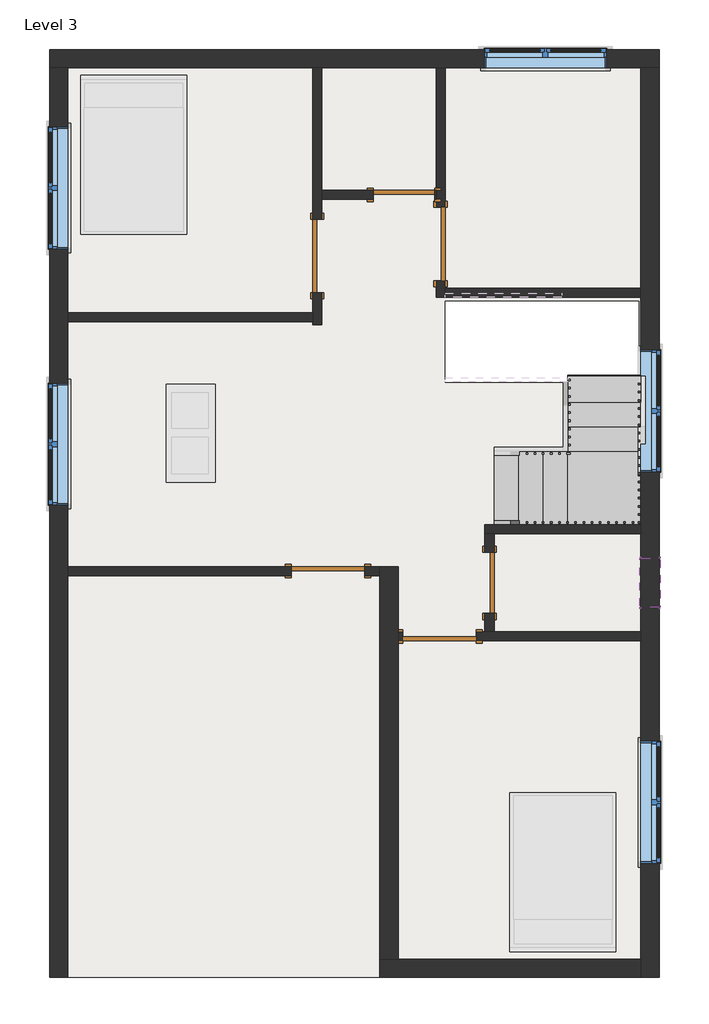
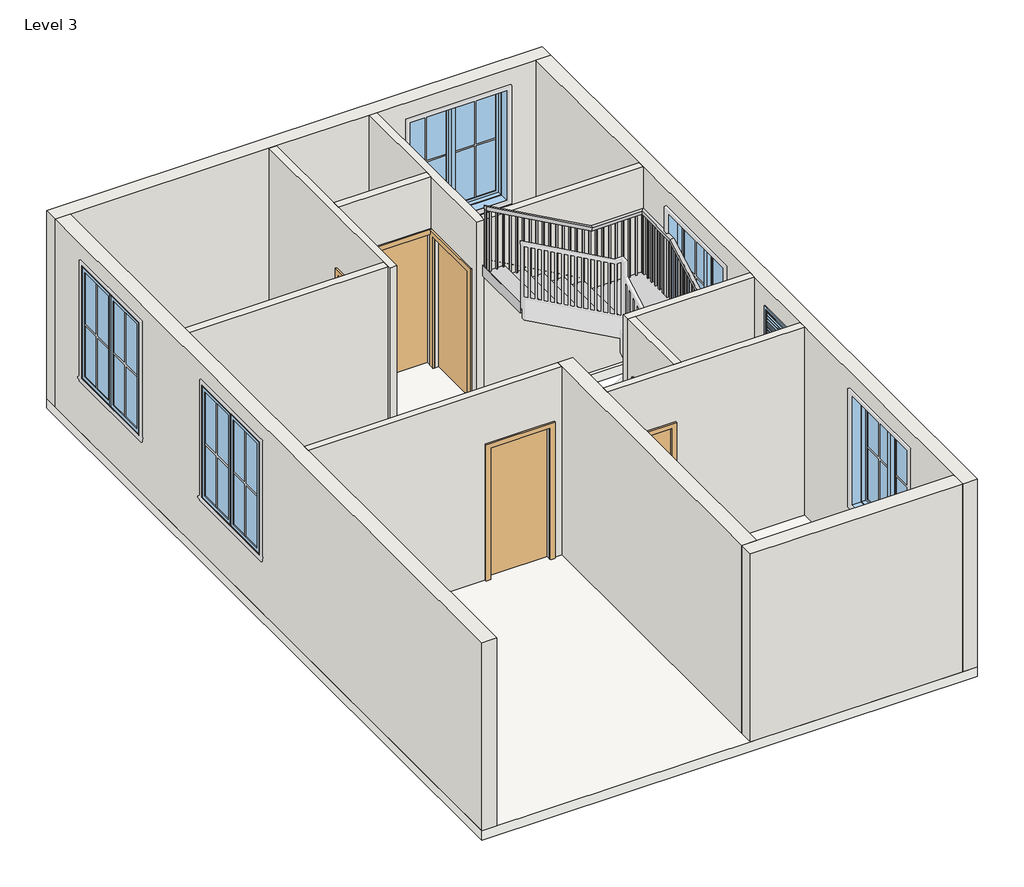
# One storey, part 1 of 2: 14 walls, 6 doors, 6 windows, 1 railing, 1 slab, 1 stair flight.
"""IFC4 building model written with IfcOpenShell, lengths in millimetres."""

from ifc_helpers import new_model, si_unit, frame, origin, place, context, project, spatial, polyline, outline, extrude, faceted_brep, transform, mapped, element, save
from components import door_214872d5, door_78caadf7, single_flush_door_3_e5f9f3c4, single_flush_door_3_305aa2a5, stair_flight_3451e034, window_casement_double_win_5_f93960c7, window_f2d8fef0

model = new_model("IFC4")

# Units and contexts
model_context = context("Model", 3, world=origin())
ifc_project = project(units=[si_unit("LENGTHUNIT", "METRE", prefix="MILLI")], contexts=[model_context])

# Site, building, storey
site = spatial("IfcSite", under=ifc_project)
building = spatial("IfcBuilding", under=site)
storey = spatial("IfcBuildingStorey", under=building, Name="Level 3", Elevation=3200.4)

# Doors
placement = place(None, origin())
door_shape = door_214872d5(model_context)
element("IfcDoor", 1, ObjectType="Single-Flush : DOOR 2'6\"", at=placement, inside=storey, context=model_context, shape_type="MappedRepresentation", body=[
    mapped(door_shape, transform((-185.4325206, 3926.3629493, 3200.4), x_axis=(1.0, 0.0, 0.0), y_axis=(0.0, 1.0, 0.0), z_axis=(0.0, 0.0, 1.0))),
])
door_2_shape = door_78caadf7(model_context)
element("IfcDoor", 2, ObjectType="Single-Flush : DOOR 2'6\"", at=placement, inside=storey, context=model_context, shape_type="MappedRepresentation", body=[
    mapped(door_2_shape, transform((881.3674794, -905.9870507, 3200.4), x_axis=(0.0, 1.0, 0.0), y_axis=(-1.0, 0.0, 0.0), z_axis=(0.0, 0.0, 1.0))),
])
single_flush_door_3_shape = single_flush_door_3_e5f9f3c4(model_context)
element("IfcDoor", 3, ObjectType="Single-Flush : DOOR 3'", at=placement, inside=storey, context=model_context, shape_type="MappedRepresentation", body=[
    mapped(single_flush_door_3_shape, transform((271.7674794, 3316.7629493, 3200.4), x_axis=(0.0, -1.0, 0.0), y_axis=(1.0, 0.0, 0.0), z_axis=(0.0, 0.0, 1.0))),
])
element("IfcDoor", 4, ObjectType="Single-Flush : DOOR 3'", at=placement, inside=storey, context=model_context, shape_type="MappedRepresentation", body=[
    mapped(single_flush_door_3_shape, transform((255.8924794, -1572.7370507, 3200.4), x_axis=(-1.0, 0.0, 0.0), y_axis=(0.0, -1.0, 0.0), z_axis=(0.0, 0.0, 1.0))),
])
single_flush_door_3_2_shape = single_flush_door_3_305aa2a5(model_context)
element("IfcDoor", 5, ObjectType="Single-Flush : DOOR 3'", at=placement, inside=storey, context=model_context, shape_type="MappedRepresentation", body=[
    mapped(single_flush_door_3_2_shape, transform((-1264.9325206, 3164.3629493, 3200.4), x_axis=(0.0, -1.0, 0.0), y_axis=(1.0, 0.0, 0.0), z_axis=(0.0, 0.0, 1.0))),
])
element("IfcDoor", 6, ObjectType="Single-Flush : DOOR 3'6\"", at=placement, inside=storey, context=model_context, shape_type="MappedRepresentation", body=[
    mapped(single_flush_door_3_shape, transform((-1131.5825206, -759.9370507, 3200.4), x_axis=(1.0, 0.0, 0.0), y_axis=(0.0, 1.0, 0.0), z_axis=(0.0, 0.0, 1.0))),
])

# Railing
element("IfcRailing", 7, ObjectType="Handrail - Rectangular", at=placement, inside=storey, context=model_context, shape_type="SolidModel", body=[
    faceted_brep([(938.5174794, -131.2870507, 4284.1333333), (938.5174794, -131.2870507, 4226.020221), (938.5174794, -182.0870507, 4226.020221), (938.5174794, -182.0870507, 4284.1333333), (2005.3174794, -131.2870507, 4876.8), (2018.4810817, -131.2870507, 4826.0), (2018.4810817, -182.0870507, 4826.0), (2005.3174794, -182.0870507, 4876.8), (2716.5174794, -131.2870507, 4876.8), (2716.5174794, -131.2870507, 4826.0), (2767.3174794, -182.0870507, 4826.0), (2767.3174794, -182.0870507, 4876.8), (2716.5174794, 579.9129493, 4876.8), (2716.5174794, 593.0765516, 4826.0), (2767.3174794, 593.0765516, 4826.0), (2767.3174794, 579.9129493, 4876.8), (2716.5174794, 1843.5629493, 5578.8277778), (2716.5174794, 1856.7265516, 5528.0277778), (2767.3174794, 1856.7265516, 5528.0277778), (2767.3174794, 1843.5629493, 5578.8277778), (2716.5174794, 2599.2129493, 5578.8277778), (2716.5174794, 2599.2129493, 5528.0277778), (2767.3174794, 2650.0129493, 5528.0277778), (2767.3174794, 2650.0129493, 5578.8277778), (1960.8674794, 2599.2129493, 5578.8277778), (1947.7038772, 2599.2129493, 5528.0277778), (1947.7038772, 2650.0129493, 5528.0277778), (1960.8674794, 2650.0129493, 5578.8277778), (328.9174794, 2599.2129493, 6485.4666667), (328.9174794, 2650.0129493, 6485.4666667), (328.9174794, 2650.0129493, 6427.3535543), (328.9174794, 2599.2129493, 6427.3535543)], [[[0, 1, 2, 3]], [[1, 0, 4, 5]], [[2, 1, 5, 6]], [[3, 2, 6, 7]], [[0, 3, 7, 4]], [[5, 4, 8, 9]], [[6, 5, 9, 10]], [[7, 6, 10, 11]], [[4, 7, 11, 8]], [[9, 8, 12, 13]], [[10, 9, 13, 14]], [[11, 10, 14, 15]], [[8, 11, 15, 12]], [[13, 12, 16, 17]], [[14, 13, 17, 18]], [[15, 14, 18, 19]], [[12, 15, 19, 16]], [[17, 16, 20, 21]], [[18, 17, 21, 22]], [[19, 18, 22, 23]], [[16, 19, 23, 20]], [[21, 20, 24, 25]], [[22, 21, 25, 26]], [[23, 22, 26, 27]], [[20, 23, 27, 24]], [[28, 29, 30, 31]], [[25, 24, 28, 31]], [[26, 25, 31, 30]], [[27, 26, 30, 29]], [[24, 27, 29, 28]]]),
    extrude(outline(polyline([(6379.7285543, 414.6424794), (6390.3118876, 395.5924794), (5401.7333333, 395.5924794), (5401.7333333, 414.6424794), (6379.7285543, 414.6424794)])), frame((0.0, 2615.0879493, 0.0), z_axis=(0.0, 1.0, 0.0), x_axis=(0.0, 0.0, 1.0)), (0.0, 0.0, 1.0), 19.05),
    extrude(outline(polyline([(6323.2841099, 516.2424794), (6333.8674432, 497.1924794), (5401.7333333, 497.1924794), (5401.7333333, 516.2424794), (6323.2841099, 516.2424794)])), frame((0.0, 2615.0879493, 0.0), z_axis=(0.0, 1.0, 0.0), x_axis=(0.0, 0.0, 1.0)), (0.0, 0.0, 1.0), 19.05),
    extrude(outline(polyline([(6266.8396654, 617.8424794), (6277.4229988, 598.7924794), (5401.7333333, 598.7924794), (5401.7333333, 617.8424794), (6266.8396654, 617.8424794)])), frame((0.0, 2615.0879493, 0.0), z_axis=(0.0, 1.0, 0.0), x_axis=(0.0, 0.0, 1.0)), (0.0, 0.0, 1.0), 19.05),
    extrude(outline(polyline([(6210.395221, 719.4424794), (6220.9785543, 700.3924794), (5232.4, 700.3924794), (5232.4, 719.4424794), (6210.395221, 719.4424794)])), frame((0.0, 2615.0879493, 0.0), z_axis=(0.0, 1.0, 0.0), x_axis=(0.0, 0.0, 1.0)), (0.0, 0.0, 1.0), 19.05),
    extrude(outline(polyline([(6153.9507765, 821.0424794), (6164.5341099, 801.9924794), (5232.4, 801.9924794), (5232.4, 821.0424794), (6153.9507765, 821.0424794)])), frame((0.0, 2615.0879493, 0.0), z_axis=(0.0, 1.0, 0.0), x_axis=(0.0, 0.0, 1.0)), (0.0, 0.0, 1.0), 19.05),
    extrude(outline(polyline([(6097.5063321, 922.6424794), (6108.0896654, 903.5924794), (5232.4, 903.5924794), (5232.4, 922.6424794), (6097.5063321, 922.6424794)])), frame((0.0, 2615.0879493, 0.0), z_axis=(0.0, 1.0, 0.0), x_axis=(0.0, 0.0, 1.0)), (0.0, 0.0, 1.0), 19.05),
    extrude(outline(polyline([(6041.0618876, 1024.2424794), (6051.645221, 1005.1924794), (5063.0666667, 1005.1924794), (5063.0666667, 1024.2424794), (6041.0618876, 1024.2424794)])), frame((0.0, 2615.0879493, 0.0), z_axis=(0.0, 1.0, 0.0), x_axis=(0.0, 0.0, 1.0)), (0.0, 0.0, 1.0), 19.05),
    extrude(outline(polyline([(5984.6174432, 1125.8424794), (5995.2007765, 1106.7924794), (5063.0666667, 1106.7924794), (5063.0666667, 1125.8424794), (5984.6174432, 1125.8424794)])), frame((0.0, 2615.0879493, 0.0), z_axis=(0.0, 1.0, 0.0), x_axis=(0.0, 0.0, 1.0)), (0.0, 0.0, 1.0), 19.05),
    extrude(outline(polyline([(5928.1729988, 1227.4424794), (5938.7563321, 1208.3924794), (5063.0666667, 1208.3924794), (5063.0666667, 1227.4424794), (5928.1729988, 1227.4424794)])), frame((0.0, 2615.0879493, 0.0), z_axis=(0.0, 1.0, 0.0), x_axis=(0.0, 0.0, 1.0)), (0.0, 0.0, 1.0), 19.05),
    extrude(outline(polyline([(5871.7285543, 1329.0424794), (5882.3118876, 1309.9924794), (4893.7333333, 1309.9924794), (4893.7333333, 1329.0424794), (5871.7285543, 1329.0424794)])), frame((0.0, 2615.0879493, 0.0), z_axis=(0.0, 1.0, 0.0), x_axis=(0.0, 0.0, 1.0)), (0.0, 0.0, 1.0), 19.05),
    extrude(outline(polyline([(5815.2841099, 1430.6424794), (5825.8674432, 1411.5924794), (4893.7333333, 1411.5924794), (4893.7333333, 1430.6424794), (5815.2841099, 1430.6424794)])), frame((0.0, 2615.0879493, 0.0), z_axis=(0.0, 1.0, 0.0), x_axis=(0.0, 0.0, 1.0)), (0.0, 0.0, 1.0), 19.05),
    extrude(outline(polyline([(5758.8396654, 1532.2424794), (5769.4229988, 1513.1924794), (4893.7333333, 1513.1924794), (4893.7333333, 1532.2424794), (5758.8396654, 1532.2424794)])), frame((0.0, 2615.0879493, 0.0), z_axis=(0.0, 1.0, 0.0), x_axis=(0.0, 0.0, 1.0)), (0.0, 0.0, 1.0), 19.05),
    extrude(outline(polyline([(5702.395221, 1633.8424794), (5712.9785543, 1614.7924794), (4724.4, 1614.7924794), (4724.4, 1633.8424794), (5702.395221, 1633.8424794)])), frame((0.0, 2615.0879493, 0.0), z_axis=(0.0, 1.0, 0.0), x_axis=(0.0, 0.0, 1.0)), (0.0, 0.0, 1.0), 19.05),
    extrude(outline(polyline([(5645.9507765, 1735.4424794), (5656.5341099, 1716.3924794), (4724.4, 1716.3924794), (4724.4, 1735.4424794), (5645.9507765, 1735.4424794)])), frame((0.0, 2615.0879493, 0.0), z_axis=(0.0, 1.0, 0.0), x_axis=(0.0, 0.0, 1.0)), (0.0, 0.0, 1.0), 19.05),
    extrude(outline(polyline([(5589.5063321, 1837.0424794), (5600.0896654, 1817.9924794), (4724.4, 1817.9924794), (4724.4, 1837.0424794), (5589.5063321, 1837.0424794)])), frame((0.0, 2615.0879493, 0.0), z_axis=(0.0, 1.0, 0.0), x_axis=(0.0, 0.0, 1.0)), (0.0, 0.0, 1.0), 19.05),
    extrude(outline(polyline([(5533.0618876, 1938.6424794), (5543.645221, 1919.5924794), (4555.0666667, 1919.5924794), (4555.0666667, 1938.6424794), (5533.0618876, 1938.6424794)])), frame((0.0, 2615.0879493, 0.0), z_axis=(0.0, 1.0, 0.0), x_axis=(0.0, 0.0, 1.0)), (0.0, 0.0, 1.0), 19.05),
    extrude(outline(polyline([(2040.2424794, 2634.1379493), (2040.2424794, 2615.0879493), (2021.1924794, 2615.0879493), (2021.1924794, 2634.1379493), (2040.2424794, 2634.1379493)])), frame((0.0, 0.0, 4555.0666667), z_axis=(0.0, 0.0, 1.0), x_axis=(1.0, 0.0, 0.0)), (0.0, 0.0, 1.0), 972.9611111),
    extrude(outline(polyline([(2141.8424794, 2634.1379493), (2141.8424794, 2615.0879493), (2122.7924794, 2615.0879493), (2122.7924794, 2634.1379493), (2141.8424794, 2634.1379493)])), frame((0.0, 0.0, 4555.0666667), z_axis=(0.0, 0.0, 1.0), x_axis=(1.0, 0.0, 0.0)), (0.0, 0.0, 1.0), 972.9611111),
    extrude(outline(polyline([(2243.4424794, 2634.1379493), (2243.4424794, 2615.0879493), (2224.3924794, 2615.0879493), (2224.3924794, 2634.1379493), (2243.4424794, 2634.1379493)])), frame((0.0, 0.0, 4555.0666667), z_axis=(0.0, 0.0, 1.0), x_axis=(1.0, 0.0, 0.0)), (0.0, 0.0, 1.0), 972.9611111),
    extrude(outline(polyline([(2345.0424794, 2634.1379493), (2345.0424794, 2615.0879493), (2325.9924794, 2615.0879493), (2325.9924794, 2634.1379493), (2345.0424794, 2634.1379493)])), frame((0.0, 0.0, 4555.0666667), z_axis=(0.0, 0.0, 1.0), x_axis=(1.0, 0.0, 0.0)), (0.0, 0.0, 1.0), 972.9611111),
    extrude(outline(polyline([(2446.6424794, 2634.1379493), (2446.6424794, 2615.0879493), (2427.5924794, 2615.0879493), (2427.5924794, 2634.1379493), (2446.6424794, 2634.1379493)])), frame((0.0, 0.0, 4555.0666667), z_axis=(0.0, 0.0, 1.0), x_axis=(1.0, 0.0, 0.0)), (0.0, 0.0, 1.0), 972.9611111),
    extrude(outline(polyline([(2548.2424794, 2634.1379493), (2548.2424794, 2615.0879493), (2529.1924794, 2615.0879493), (2529.1924794, 2634.1379493), (2548.2424794, 2634.1379493)])), frame((0.0, 0.0, 4555.0666667), z_axis=(0.0, 0.0, 1.0), x_axis=(1.0, 0.0, 0.0)), (0.0, 0.0, 1.0), 972.9611111),
    extrude(outline(polyline([(2649.8424794, 2634.1379493), (2649.8424794, 2615.0879493), (2630.7924794, 2615.0879493), (2630.7924794, 2634.1379493), (2649.8424794, 2634.1379493)])), frame((0.0, 0.0, 4555.0666667), z_axis=(0.0, 0.0, 1.0), x_axis=(1.0, 0.0, 0.0)), (0.0, 0.0, 1.0), 972.9611111),
    extrude(outline(polyline([(2751.4424794, 2576.9879493), (2732.3924794, 2576.9879493), (2732.3924794, 2596.0379493), (2751.4424794, 2596.0379493), (2751.4424794, 2576.9879493)])), frame((0.0, 0.0, 4555.0666667), z_axis=(0.0, 0.0, 1.0), x_axis=(1.0, 0.0, 0.0)), (0.0, 0.0, 1.0), 972.9611111),
    extrude(outline(polyline([(2751.4424794, 2475.3879493), (2732.3924794, 2475.3879493), (2732.3924794, 2494.4379493), (2751.4424794, 2494.4379493), (2751.4424794, 2475.3879493)])), frame((0.0, 0.0, 4555.0666667), z_axis=(0.0, 0.0, 1.0), x_axis=(1.0, 0.0, 0.0)), (0.0, 0.0, 1.0), 972.9611111),
    extrude(outline(polyline([(2751.4424794, 2373.7879493), (2732.3924794, 2373.7879493), (2732.3924794, 2392.8379493), (2751.4424794, 2392.8379493), (2751.4424794, 2373.7879493)])), frame((0.0, 0.0, 4555.0666667), z_axis=(0.0, 0.0, 1.0), x_axis=(1.0, 0.0, 0.0)), (0.0, 0.0, 1.0), 972.9611111),
    extrude(outline(polyline([(2751.4424794, 2272.1879493), (2732.3924794, 2272.1879493), (2732.3924794, 2291.2379493), (2751.4424794, 2291.2379493), (2751.4424794, 2272.1879493)])), frame((0.0, 0.0, 4555.0666667), z_axis=(0.0, 0.0, 1.0), x_axis=(1.0, 0.0, 0.0)), (0.0, 0.0, 1.0), 972.9611111),
    extrude(outline(polyline([(2751.4424794, 2170.5879493), (2732.3924794, 2170.5879493), (2732.3924794, 2189.6379493), (2751.4424794, 2189.6379493), (2751.4424794, 2170.5879493)])), frame((0.0, 0.0, 4555.0666667), z_axis=(0.0, 0.0, 1.0), x_axis=(1.0, 0.0, 0.0)), (0.0, 0.0, 1.0), 972.9611111),
    extrude(outline(polyline([(2751.4424794, 2068.9879493), (2732.3924794, 2068.9879493), (2732.3924794, 2088.0379493), (2751.4424794, 2088.0379493), (2751.4424794, 2068.9879493)])), frame((0.0, 0.0, 4555.0666667), z_axis=(0.0, 0.0, 1.0), x_axis=(1.0, 0.0, 0.0)), (0.0, 0.0, 1.0), 972.9611111),
    extrude(outline(polyline([(2751.4424794, 1967.3879493), (2732.3924794, 1967.3879493), (2732.3924794, 1986.4379493), (2751.4424794, 1986.4379493), (2751.4424794, 1967.3879493)])), frame((0.0, 0.0, 4555.0666667), z_axis=(0.0, 0.0, 1.0), x_axis=(1.0, 0.0, 0.0)), (0.0, 0.0, 1.0), 972.9611111),
    extrude(outline(polyline([(2751.4424794, 1865.7879493), (2732.3924794, 1865.7879493), (2732.3924794, 1884.8379493), (2751.4424794, 1884.8379493), (2751.4424794, 1865.7879493)])), frame((0.0, 0.0, 4555.0666667), z_axis=(0.0, 0.0, 1.0), x_axis=(1.0, 0.0, 0.0)), (0.0, 0.0, 1.0), 972.9611111),
    extrude(outline(polyline([(1764.1879493, 5476.6174432), (1783.2379493, 5487.2007765), (1783.2379493, 4555.0666667), (1764.1879493, 4555.0666667), (1764.1879493, 5476.6174432)])), frame((2732.3924794, 0.0, 0.0), z_axis=(1.0, 0.0, 0.0), x_axis=(0.0, 1.0, 0.0)), (0.0, 0.0, 1.0), 19.05),
    extrude(outline(polyline([(1662.5879493, 5420.1729988), (1681.6379493, 5430.7563321), (1681.6379493, 4555.0666667), (1662.5879493, 4555.0666667), (1662.5879493, 5420.1729988)])), frame((2732.3924794, 0.0, 0.0), z_axis=(1.0, 0.0, 0.0), x_axis=(0.0, 1.0, 0.0)), (0.0, 0.0, 1.0), 19.05),
    extrude(outline(polyline([(1560.9879493, 5363.7285543), (1580.0379493, 5374.3118876), (1580.0379493, 4385.7333333), (1560.9879493, 4385.7333333), (1560.9879493, 5363.7285543)])), frame((2732.3924794, 0.0, 0.0), z_axis=(1.0, 0.0, 0.0), x_axis=(0.0, 1.0, 0.0)), (0.0, 0.0, 1.0), 19.05),
    extrude(outline(polyline([(1459.3879493, 5307.2841099), (1478.4379493, 5317.8674432), (1478.4379493, 4385.7333333), (1459.3879493, 4385.7333333), (1459.3879493, 5307.2841099)])), frame((2732.3924794, 0.0, 0.0), z_axis=(1.0, 0.0, 0.0), x_axis=(0.0, 1.0, 0.0)), (0.0, 0.0, 1.0), 19.05),
    extrude(outline(polyline([(1357.7879493, 5250.8396654), (1376.8379493, 5261.4229988), (1376.8379493, 4385.7333333), (1357.7879493, 4385.7333333), (1357.7879493, 5250.8396654)])), frame((2732.3924794, 0.0, 0.0), z_axis=(1.0, 0.0, 0.0), x_axis=(0.0, 1.0, 0.0)), (0.0, 0.0, 1.0), 19.05),
    extrude(outline(polyline([(1256.1879493, 5194.395221), (1275.2379493, 5204.9785543), (1275.2379493, 4216.4), (1256.1879493, 4216.4), (1256.1879493, 5194.395221)])), frame((2732.3924794, 0.0, 0.0), z_axis=(1.0, 0.0, 0.0), x_axis=(0.0, 1.0, 0.0)), (0.0, 0.0, 1.0), 19.05),
    extrude(outline(polyline([(1154.5879493, 5137.9507765), (1173.6379493, 5148.5341099), (1173.6379493, 4216.4), (1154.5879493, 4216.4), (1154.5879493, 5137.9507765)])), frame((2732.3924794, 0.0, 0.0), z_axis=(1.0, 0.0, 0.0), x_axis=(0.0, 1.0, 0.0)), (0.0, 0.0, 1.0), 19.05),
    extrude(outline(polyline([(1052.9879493, 5081.5063321), (1072.0379493, 5092.0896654), (1072.0379493, 4216.4), (1052.9879493, 4216.4), (1052.9879493, 5081.5063321)])), frame((2732.3924794, 0.0, 0.0), z_axis=(1.0, 0.0, 0.0), x_axis=(0.0, 1.0, 0.0)), (0.0, 0.0, 1.0), 19.05),
    extrude(outline(polyline([(951.3879493, 5025.0618876), (970.4379493, 5035.645221), (970.4379493, 4047.0666667), (951.3879493, 4047.0666667), (951.3879493, 5025.0618876)])), frame((2732.3924794, 0.0, 0.0), z_axis=(1.0, 0.0, 0.0), x_axis=(0.0, 1.0, 0.0)), (0.0, 0.0, 1.0), 19.05),
    extrude(outline(polyline([(849.7879493, 4968.6174432), (868.8379493, 4979.2007765), (868.8379493, 4047.0666667), (849.7879493, 4047.0666667), (849.7879493, 4968.6174432)])), frame((2732.3924794, 0.0, 0.0), z_axis=(1.0, 0.0, 0.0), x_axis=(0.0, 1.0, 0.0)), (0.0, 0.0, 1.0), 19.05),
    extrude(outline(polyline([(748.1879493, 4912.1729988), (767.2379493, 4922.7563321), (767.2379493, 4047.0666667), (748.1879493, 4047.0666667), (748.1879493, 4912.1729988)])), frame((2732.3924794, 0.0, 0.0), z_axis=(1.0, 0.0, 0.0), x_axis=(0.0, 1.0, 0.0)), (0.0, 0.0, 1.0), 19.05),
    extrude(outline(polyline([(646.5879493, 4855.7285543), (665.6379493, 4866.3118876), (665.6379493, 3877.7333333), (646.5879493, 3877.7333333), (646.5879493, 4855.7285543)])), frame((2732.3924794, 0.0, 0.0), z_axis=(1.0, 0.0, 0.0), x_axis=(0.0, 1.0, 0.0)), (0.0, 0.0, 1.0), 19.05),
    extrude(outline(polyline([(2751.4424794, 544.9879493), (2732.3924794, 544.9879493), (2732.3924794, 564.0379493), (2751.4424794, 564.0379493), (2751.4424794, 544.9879493)])), frame((0.0, 0.0, 3877.7333333), z_axis=(0.0, 0.0, 1.0), x_axis=(1.0, 0.0, 0.0)), (0.0, 0.0, 1.0), 948.2666667),
    extrude(outline(polyline([(2751.4424794, 443.3879493), (2732.3924794, 443.3879493), (2732.3924794, 462.4379493), (2751.4424794, 462.4379493), (2751.4424794, 443.3879493)])), frame((0.0, 0.0, 3877.7333333), z_axis=(0.0, 0.0, 1.0), x_axis=(1.0, 0.0, 0.0)), (0.0, 0.0, 1.0), 948.2666667),
    extrude(outline(polyline([(2751.4424794, 341.7879493), (2732.3924794, 341.7879493), (2732.3924794, 360.8379493), (2751.4424794, 360.8379493), (2751.4424794, 341.7879493)])), frame((0.0, 0.0, 3877.7333333), z_axis=(0.0, 0.0, 1.0), x_axis=(1.0, 0.0, 0.0)), (0.0, 0.0, 1.0), 948.2666667),
    extrude(outline(polyline([(2751.4424794, 240.1879493), (2732.3924794, 240.1879493), (2732.3924794, 259.2379493), (2751.4424794, 259.2379493), (2751.4424794, 240.1879493)])), frame((0.0, 0.0, 3877.7333333), z_axis=(0.0, 0.0, 1.0), x_axis=(1.0, 0.0, 0.0)), (0.0, 0.0, 1.0), 948.2666667),
    extrude(outline(polyline([(2751.4424794, 138.5879493), (2732.3924794, 138.5879493), (2732.3924794, 157.6379493), (2751.4424794, 157.6379493), (2751.4424794, 138.5879493)])), frame((0.0, 0.0, 3877.7333333), z_axis=(0.0, 0.0, 1.0), x_axis=(1.0, 0.0, 0.0)), (0.0, 0.0, 1.0), 948.2666667),
    extrude(outline(polyline([(2751.4424794, 36.9879493), (2732.3924794, 36.9879493), (2732.3924794, 56.0379493), (2751.4424794, 56.0379493), (2751.4424794, 36.9879493)])), frame((0.0, 0.0, 3877.7333333), z_axis=(0.0, 0.0, 1.0), x_axis=(1.0, 0.0, 0.0)), (0.0, 0.0, 1.0), 948.2666667),
    extrude(outline(polyline([(2751.4424794, -64.6120507), (2732.3924794, -64.6120507), (2732.3924794, -45.5620507), (2751.4424794, -45.5620507), (2751.4424794, -64.6120507)])), frame((0.0, 0.0, 3877.7333333), z_axis=(0.0, 0.0, 1.0), x_axis=(1.0, 0.0, 0.0)), (0.0, 0.0, 1.0), 948.2666667),
    extrude(outline(polyline([(2656.1924794, -166.2120507), (2656.1924794, -147.1620507), (2675.2424794, -147.1620507), (2675.2424794, -166.2120507), (2656.1924794, -166.2120507)])), frame((0.0, 0.0, 3877.7333333), z_axis=(0.0, 0.0, 1.0), x_axis=(1.0, 0.0, 0.0)), (0.0, 0.0, 1.0), 948.2666667),
    extrude(outline(polyline([(2554.5924794, -166.2120507), (2554.5924794, -147.1620507), (2573.6424794, -147.1620507), (2573.6424794, -166.2120507), (2554.5924794, -166.2120507)])), frame((0.0, 0.0, 3877.7333333), z_axis=(0.0, 0.0, 1.0), x_axis=(1.0, 0.0, 0.0)), (0.0, 0.0, 1.0), 948.2666667),
    extrude(outline(polyline([(2452.9924794, -166.2120507), (2452.9924794, -147.1620507), (2472.0424794, -147.1620507), (2472.0424794, -166.2120507), (2452.9924794, -166.2120507)])), frame((0.0, 0.0, 3877.7333333), z_axis=(0.0, 0.0, 1.0), x_axis=(1.0, 0.0, 0.0)), (0.0, 0.0, 1.0), 948.2666667),
    extrude(outline(polyline([(2351.3924794, -166.2120507), (2351.3924794, -147.1620507), (2370.4424794, -147.1620507), (2370.4424794, -166.2120507), (2351.3924794, -166.2120507)])), frame((0.0, 0.0, 3877.7333333), z_axis=(0.0, 0.0, 1.0), x_axis=(1.0, 0.0, 0.0)), (0.0, 0.0, 1.0), 948.2666667),
    extrude(outline(polyline([(2249.7924794, -166.2120507), (2249.7924794, -147.1620507), (2268.8424794, -147.1620507), (2268.8424794, -166.2120507), (2249.7924794, -166.2120507)])), frame((0.0, 0.0, 3877.7333333), z_axis=(0.0, 0.0, 1.0), x_axis=(1.0, 0.0, 0.0)), (0.0, 0.0, 1.0), 948.2666667),
    extrude(outline(polyline([(2148.1924794, -166.2120507), (2148.1924794, -147.1620507), (2167.2424794, -147.1620507), (2167.2424794, -166.2120507), (2148.1924794, -166.2120507)])), frame((0.0, 0.0, 3877.7333333), z_axis=(0.0, 0.0, 1.0), x_axis=(1.0, 0.0, 0.0)), (0.0, 0.0, 1.0), 948.2666667),
    extrude(outline(polyline([(2046.5924794, -166.2120507), (2046.5924794, -147.1620507), (2065.6424794, -147.1620507), (2065.6424794, -166.2120507), (2046.5924794, -166.2120507)])), frame((0.0, 0.0, 3877.7333333), z_axis=(0.0, 0.0, 1.0), x_axis=(1.0, 0.0, 0.0)), (0.0, 0.0, 1.0), 948.2666667),
    extrude(outline(polyline([(4795.7563321, 1964.0424794), (4785.1729988, 1944.9924794), (3877.7333333, 1944.9924794), (3877.7333333, 1964.0424794), (4795.7563321, 1964.0424794)])), frame((0.0, -166.2120507, 0.0), z_axis=(0.0, 1.0, 0.0), x_axis=(0.0, 0.0, 1.0)), (0.0, 0.0, 1.0), 19.05),
    extrude(outline(polyline([(4739.3118876, 1862.4424794), (4728.7285543, 1843.3924794), (3877.7333333, 1843.3924794), (3877.7333333, 1862.4424794), (4739.3118876, 1862.4424794)])), frame((0.0, -166.2120507, 0.0), z_axis=(0.0, 1.0, 0.0), x_axis=(0.0, 0.0, 1.0)), (0.0, 0.0, 1.0), 19.05),
    extrude(outline(polyline([(4682.8674432, 1760.8424794), (4672.2841099, 1741.7924794), (3708.4, 1741.7924794), (3708.4, 1760.8424794), (4682.8674432, 1760.8424794)])), frame((0.0, -166.2120507, 0.0), z_axis=(0.0, 1.0, 0.0), x_axis=(0.0, 0.0, 1.0)), (0.0, 0.0, 1.0), 19.05),
    extrude(outline(polyline([(4626.4229988, 1659.2424794), (4615.8396654, 1640.1924794), (3708.4, 1640.1924794), (3708.4, 1659.2424794), (4626.4229988, 1659.2424794)])), frame((0.0, -166.2120507, 0.0), z_axis=(0.0, 1.0, 0.0), x_axis=(0.0, 0.0, 1.0)), (0.0, 0.0, 1.0), 19.05),
    extrude(outline(polyline([(4569.9785543, 1557.6424794), (4559.395221, 1538.5924794), (3708.4, 1538.5924794), (3708.4, 1557.6424794), (4569.9785543, 1557.6424794)])), frame((0.0, -166.2120507, 0.0), z_axis=(0.0, 1.0, 0.0), x_axis=(0.0, 0.0, 1.0)), (0.0, 0.0, 1.0), 19.05),
    extrude(outline(polyline([(4513.5341099, 1456.0424794), (4502.9507765, 1436.9924794), (3539.0666667, 1436.9924794), (3539.0666667, 1456.0424794), (4513.5341099, 1456.0424794)])), frame((0.0, -166.2120507, 0.0), z_axis=(0.0, 1.0, 0.0), x_axis=(0.0, 0.0, 1.0)), (0.0, 0.0, 1.0), 19.05),
    extrude(outline(polyline([(4457.0896654, 1354.4424794), (4446.5063321, 1335.3924794), (3539.0666667, 1335.3924794), (3539.0666667, 1354.4424794), (4457.0896654, 1354.4424794)])), frame((0.0, -166.2120507, 0.0), z_axis=(0.0, 1.0, 0.0), x_axis=(0.0, 0.0, 1.0)), (0.0, 0.0, 1.0), 19.05),
    extrude(outline(polyline([(4400.645221, 1252.8424794), (4390.0618876, 1233.7924794), (3539.0666667, 1233.7924794), (3539.0666667, 1252.8424794), (4400.645221, 1252.8424794)])), frame((0.0, -166.2120507, 0.0), z_axis=(0.0, 1.0, 0.0), x_axis=(0.0, 0.0, 1.0)), (0.0, 0.0, 1.0), 19.05),
    extrude(outline(polyline([(4344.2007765, 1151.2424794), (4333.6174432, 1132.1924794), (3369.7333333, 1132.1924794), (3369.7333333, 1151.2424794), (4344.2007765, 1151.2424794)])), frame((0.0, -166.2120507, 0.0), z_axis=(0.0, 1.0, 0.0), x_axis=(0.0, 0.0, 1.0)), (0.0, 0.0, 1.0), 19.05),
    extrude(outline(polyline([(4287.7563321, 1049.6424794), (4277.1729988, 1030.5924794), (3369.7333333, 1030.5924794), (3369.7333333, 1049.6424794), (4287.7563321, 1049.6424794)])), frame((0.0, -166.2120507, 0.0), z_axis=(0.0, 1.0, 0.0), x_axis=(0.0, 0.0, 1.0)), (0.0, 0.0, 1.0), 19.05),
    extrude(outline(polyline([(2751.4424794, 2615.0879493), (2732.3924794, 2615.0879493), (2732.3924794, 2634.1379493), (2751.4424794, 2634.1379493), (2751.4424794, 2615.0879493)])), frame((0.0, 0.0, 4555.0666667), z_axis=(0.0, 0.0, 1.0), x_axis=(1.0, 0.0, 0.0)), (0.0, 0.0, 1.0), 972.9611111),
    extrude(outline(polyline([(2732.3924794, -166.2120507), (2732.3924794, -147.1620507), (2751.4424794, -147.1620507), (2751.4424794, -166.2120507), (2732.3924794, -166.2120507)])), frame((0.0, 0.0, 3877.7333333), z_axis=(0.0, 0.0, 1.0), x_axis=(1.0, 0.0, 0.0)), (0.0, 0.0, 1.0), 948.2666667),
    extrude(outline(polyline([(6416.770221, 347.9674794), (6427.3535543, 328.9174794), (5401.7333333, 328.9174794), (5401.7333333, 347.9674794), (6416.770221, 347.9674794)])), frame((0.0, 2615.0879493, 0.0), z_axis=(0.0, 1.0, 0.0), x_axis=(0.0, 0.0, 1.0)), (0.0, 0.0, 1.0), 19.05),
    extrude(outline(polyline([(4236.6035543, 957.5674794), (4226.020221, 938.5174794), (3369.7333333, 938.5174794), (3369.7333333, 957.5674794), (4236.6035543, 957.5674794)])), frame((0.0, -166.2120507, 0.0), z_axis=(0.0, 1.0, 0.0), x_axis=(0.0, 0.0, 1.0)), (0.0, 0.0, 1.0), 19.05),
])

# Slab
element("IfcSlab", 8, ObjectType="FLOOR 6\"", at=placement, inside=storey, context=model_context, shape_type="SweptSolid", body=[
    extrude(outline(polyline([(2995.9174794, 5736.1129493), (2995.9174794, -5820.8870507), (-4598.6825206, -5820.8870507), (-4598.6825206, 5736.1129493), (2995.9174794, 5736.1129493)]), holes=[polyline([(2741.9174794, -156.6870507), (2741.9174794, 2599.2129493), (328.9174794, 2599.2129493), (328.9174794, 1595.9129493), (1802.1174794, 1595.9129493), (1802.1174794, 706.9129493), (1040.1174794, 706.9129493), (1040.1174794, -156.6870507), (2741.9174794, -156.6870507)])]), frame((0.0, 0.0, 3048.0), z_axis=(0.0, 0.0, 1.0), x_axis=(1.0, 0.0, 0.0)), (0.0, 0.0, 1.0), 152.4),
])

# Stair flight
stair_flight_shape = stair_flight_3451e034(model_context)
element("IfcStairFlight", 9, ObjectType="2\" Tread 1\" Nosing 1/4\" Riser", at=placement, inside=storey, context=model_context, shape_type="MappedRepresentation", body=[
    mapped(stair_flight_shape, transform((0.0, 0.0, 0.0), x_axis=(1.0, 0.0, 0.0), y_axis=(0.0, 1.0, 0.0), z_axis=(0.0, 0.0, 1.0))),
])

# Walls
element("IfcWall", 10, at=placement, inside=storey, context=model_context, shape_type="Brep", body=[
    faceted_brep([(-1322.0825206, 2707.1629493, 5334.0), (-1322.0825206, 2707.1629493, 3200.4), (-1322.0825206, 2459.5129493, 3200.4), (-1322.0825206, 2345.2129493, 3200.4), (-1322.0825206, 2307.1129493, 3200.4), (-1322.0825206, 2307.1129493, 6248.4), (-1322.0825206, 2345.2129493, 6248.4), (-1322.0825206, 2459.5129493, 6248.4), (-1322.0825206, 5507.5129493, 6248.4), (-1322.0825206, 5507.5129493, 3200.4), (-1322.0825206, 3621.5629493, 3200.4), (-1322.0825206, 3621.5629493, 5334.0), (-1207.7825206, 2307.1129493, 3200.4), (-1207.7825206, 2707.1629493, 3200.4), (-1207.7825206, 2707.1629493, 5334.0), (-1207.7825206, 3621.5629493, 5334.0), (-1207.7825206, 3621.5629493, 3200.4), (-1207.7825206, 3869.2129493, 3200.4), (-1207.7825206, 3983.5129493, 3200.4), (-1207.7825206, 5507.5129493, 3200.4), (-1207.7825206, 5507.5129493, 6248.4), (-1207.7825206, 3983.5129493, 6248.4), (-1207.7825206, 3869.2129493, 6248.4), (-1207.7825206, 2307.1129493, 6248.4)], [[[0, 1, 2, 3, 4, 5, 6, 7, 8, 9, 10, 11]], [[12, 13, 14, 15, 16, 17, 18, 19, 20, 21, 22, 23]], [[10, 9, 19, 18, 17, 16]], [[4, 3, 2, 1, 13, 12]], [[5, 4, 12, 23]], [[9, 8, 20, 19]], [[14, 13, 1, 0]], [[15, 14, 0, 11]], [[16, 15, 11, 10]], [[8, 7, 6, 5, 23, 22, 21, 20]]]),
])
element("IfcWall", 11, at=placement, inside=storey, context=model_context, shape_type="SweptSolid", body=[
    extrude(outline(polyline([(-1322.0825206, 2345.2129493), (-4370.0825206, 2345.2129493), (-4370.0825206, 2459.5129493), (-1322.0825206, 2459.5129493), (-1322.0825206, 2345.2129493)])), frame((0.0, 0.0, 3200.4), z_axis=(0.0, 0.0, 1.0), x_axis=(1.0, 0.0, 0.0)), (0.0, 0.0, 1.0), 3048.0),
])
element("IfcWall", 12, at=placement, inside=storey, context=model_context, shape_type="SweptSolid", body=[
    extrude(outline(polyline([(5334.0, 195.5674794), (3200.4, 195.5674794), (3200.4, 214.6174794), (6248.4, 214.6174794), (6248.4, -1207.7825206), (3200.4, -1207.7825206), (3200.4, -566.4325206), (5334.0, -566.4325206), (5334.0, 195.5674794)])), frame((0.0, 3869.2129493, 0.0), z_axis=(0.0, 1.0, 0.0), x_axis=(0.0, 0.0, 1.0)), (0.0, 0.0, 1.0), 114.3),
])
element("IfcWall", 13, at=placement, inside=storey, context=model_context, shape_type="Brep", body=[
    faceted_brep([(214.6174794, 2859.5629493, 5334.0), (214.6174794, 2859.5629493, 3200.4), (214.6174794, 2650.0129493, 3200.4), (214.6174794, 2650.0129493, 6248.4), (214.6174794, 3869.2129493, 6248.4), (214.6174794, 3983.5129493, 6248.4), (214.6174794, 5507.5129493, 6248.4), (214.6174794, 5507.5129493, 3200.4), (214.6174794, 3983.5129493, 3200.4), (214.6174794, 3869.2129493, 3200.4), (214.6174794, 3773.9629493, 3200.4), (214.6174794, 3773.9629493, 5334.0), (328.9174794, 2650.0129493, 3200.4), (328.9174794, 2764.3129493, 3200.4), (328.9174794, 2859.5629493, 3200.4), (328.9174794, 2859.5629493, 5334.0), (328.9174794, 3773.9629493, 5334.0), (328.9174794, 3773.9629493, 3200.4), (328.9174794, 5507.5129493, 3200.4), (328.9174794, 5507.5129493, 6248.4), (328.9174794, 2764.3129493, 6248.4), (328.9174794, 2650.0129493, 6248.4)], [[[0, 1, 2, 3, 4, 5, 6, 7, 8, 9, 10, 11]], [[12, 13, 14, 15, 16, 17, 18, 19, 20, 21]], [[2, 1, 14, 13, 12]], [[10, 9, 8, 7, 18, 17]], [[7, 6, 19, 18]], [[3, 2, 12, 21]], [[15, 14, 1, 0]], [[16, 15, 0, 11]], [[17, 16, 11, 10]], [[6, 5, 4, 3, 21, 20, 19]]]),
])
element("IfcWall", 14, at=placement, inside=storey, context=model_context, shape_type="SweptSolid", body=[
    extrude(outline(polyline([(2767.3174794, 2650.0129493), (328.9174794, 2650.0129493), (328.9174794, 2764.3129493), (2767.3174794, 2764.3129493), (2767.3174794, 2650.0129493)])), frame((0.0, 0.0, 3200.4), z_axis=(0.0, 0.0, 1.0), x_axis=(1.0, 0.0, 0.0)), (0.0, 0.0, 1.0), 3048.0),
])
element("IfcWall", 15, at=placement, inside=storey, context=model_context, shape_type="Brep", body=[
    faceted_brep([(2767.3174794, -182.0870507, 3200.4), (824.2174794, -182.0870507, 3200.4), (824.2174794, -182.0870507, 6248.4), (2767.3174794, -182.0870507, 6248.4), (2767.3174794, -296.3870507, 3200.4), (2767.3174794, -296.3870507, 6248.4), (938.5174794, -296.3870507, 6248.4), (824.2174794, -296.3870507, 6248.4), (824.2174794, -296.3870507, 3200.4), (938.5174794, -296.3870507, 3200.4)], [[[0, 1, 2, 3]], [[4, 5, 6, 7, 8, 9]], [[1, 0, 4, 9, 8]], [[0, 3, 5, 4]], [[2, 1, 8, 7]], [[3, 2, 7, 6, 5]]]),
])
element("IfcWall", 16, at=placement, inside=storey, context=model_context, shape_type="SweptSolid", body=[
    extrude(outline(polyline([(-296.3870507, 3200.4), (-524.9870507, 3200.4), (-524.9870507, 5334.0), (-1286.9870507, 5334.0), (-1286.9870507, 3200.4), (-1515.5870507, 3200.4), (-1515.5870507, 6248.4), (-296.3870507, 6248.4), (-296.3870507, 3200.4)])), frame((824.2174794, 0.0, 0.0), z_axis=(1.0, 0.0, 0.0), x_axis=(0.0, 1.0, 0.0)), (0.0, 0.0, 1.0), 114.3),
])
element("IfcWall", 17, at=placement, inside=storey, context=model_context, shape_type="Brep", body=[
    faceted_brep([(-201.3075206, -1515.5870507, 5334.0), (-201.3075206, -1515.5870507, 3200.4), (-255.2825206, -1515.5870507, 3200.4), (-255.2825206, -1515.5870507, 6248.4), (824.2174794, -1515.5870507, 6248.4), (938.5174794, -1515.5870507, 6248.4), (2767.3174794, -1515.5870507, 6248.4), (2767.3174794, -1515.5870507, 3200.4), (938.5174794, -1515.5870507, 3200.4), (824.2174794, -1515.5870507, 3200.4), (713.0924794, -1515.5870507, 3200.4), (713.0924794, -1515.5870507, 5334.0), (-255.2825206, -1629.8870507, 3200.4), (-201.3075206, -1629.8870507, 3200.4), (-201.3075206, -1629.8870507, 5334.0), (713.0924794, -1629.8870507, 5334.0), (713.0924794, -1629.8870507, 3200.4), (2767.3174794, -1629.8870507, 3200.4), (2767.3174794, -1629.8870507, 6248.4), (-255.2825206, -1629.8870507, 6248.4)], [[[0, 1, 2, 3, 4, 5, 6, 7, 8, 9, 10, 11]], [[12, 13, 14, 15, 16, 17, 18, 19]], [[2, 1, 13, 12]], [[10, 9, 8, 7, 17, 16]], [[7, 6, 18, 17]], [[3, 2, 12, 19]], [[14, 13, 1, 0]], [[15, 14, 0, 11]], [[16, 15, 11, 10]], [[6, 5, 4, 3, 19, 18]]]),
])
element("IfcWall", 18, at=placement, inside=storey, context=model_context, shape_type="SweptSolid", body=[
    extrude(outline(polyline([(5334.0, -674.3825206), (3200.4, -674.3825206), (3200.4, -483.8825206), (6248.4, -483.8825206), (6248.4, -4370.0825206), (3200.4, -4370.0825206), (3200.4, -1588.7825206), (5334.0, -1588.7825206), (5334.0, -674.3825206)])), frame((0.0, -817.0870507, 0.0), z_axis=(0.0, 1.0, 0.0), x_axis=(0.0, 0.0, 1.0)), (0.0, 0.0, 1.0), 114.3),
])
element("IfcWall", 19, ObjectType="WALL 9\"", at=placement, inside=storey, context=model_context, shape_type="Brep", body=[
    faceted_brep([(-4598.6825206, 5507.5129493, 3200.4), (-4370.0825206, 5507.5129493, 3200.4), (-1322.0825206, 5507.5129493, 3200.4), (-1207.7825206, 5507.5129493, 3200.4), (214.6174794, 5507.5129493, 3200.4), (328.9174794, 5507.5129493, 3200.4), (2767.3174794, 5507.5129493, 3200.4), (2995.9174794, 5507.5129493, 3200.4), (2995.9174794, 5507.5129493, 6248.4), (2767.3174794, 5507.5129493, 6248.4), (328.9174794, 5507.5129493, 6248.4), (214.6174794, 5507.5129493, 6248.4), (-1207.7825206, 5507.5129493, 6248.4), (-1322.0825206, 5507.5129493, 6248.4), (-4370.0825206, 5507.5129493, 6248.4), (-4598.6825206, 5507.5129493, 6248.4), (2338.6924794, 5507.5129493, 5943.6), (2338.6924794, 5507.5129493, 4114.8), (814.6924794, 5507.5129493, 4114.8), (814.6924794, 5507.5129493, 5943.6), (-4598.6825206, 5736.1129493, 3200.4), (-4598.6825206, 5736.1129493, 6248.4), (2995.9174794, 5736.1129493, 6248.4), (2995.9174794, 5736.1129493, 3200.4), (2338.6924794, 5736.1129493, 5943.6), (814.6924794, 5736.1129493, 5943.6), (814.6924794, 5736.1129493, 4114.8), (2338.6924794, 5736.1129493, 4114.8)], [[[0, 1, 2, 3, 4, 5, 6, 7, 8, 9, 10, 11, 12, 13, 14, 15], [16, 17, 18, 19]], [[20, 21, 22, 23], [24, 25, 26, 27]], [[7, 6, 5, 4, 3, 2, 1, 0, 20, 23]], [[8, 7, 23, 22]], [[0, 15, 21, 20]], [[17, 16, 24, 27]], [[18, 17, 27, 26]], [[19, 18, 26, 25]], [[16, 19, 25, 24]], [[15, 14, 13, 12, 11, 10, 9, 8, 22, 21]]]),
])
element("IfcWall", 20, ObjectType="WALL 9\"", at=placement, inside=storey, context=model_context, shape_type="Brep", body=[
    faceted_brep([(2767.3174794, 5507.5129493, 3200.4), (2767.3174794, 2764.3129493, 3200.4), (2767.3174794, 2650.0129493, 3200.4), (2767.3174794, -182.0870507, 3200.4), (2767.3174794, -296.3870507, 3200.4), (2767.3174794, -1515.5870507, 3200.4), (2767.3174794, -1629.8870507, 3200.4), (2767.3174794, -5592.2870507, 3200.4), (2767.3174794, -5820.8870507, 3200.4), (2767.3174794, -5820.8870507, 6248.4), (2767.3174794, -5592.2870507, 6248.4), (2767.3174794, -1629.8870507, 6248.4), (2767.3174794, -1515.5870507, 6248.4), (2767.3174794, -296.3870507, 6248.4), (2767.3174794, -182.0870507, 6248.4), (2767.3174794, 2650.0129493, 6248.4), (2767.3174794, 2764.3129493, 6248.4), (2767.3174794, 5507.5129493, 6248.4), (2767.3174794, 471.9629493, 5943.6), (2767.3174794, 471.9629493, 4114.8), (2767.3174794, 1995.9629493, 4114.8), (2767.3174794, 1995.9629493, 5943.6), (2767.3174794, -4401.6620507, 5943.6), (2767.3174794, -4401.6620507, 4114.8), (2767.3174794, -2877.6620507, 4114.8), (2767.3174794, -2877.6620507, 5943.6), (2767.3174794, -1210.7870507, 5943.6), (2767.3174794, -1210.7870507, 5334.0), (2767.3174794, -601.1870507, 5334.0), (2767.3174794, -601.1870507, 5943.6), (2995.9174794, 5507.5129493, 3200.4), (2995.9174794, 5507.5129493, 6248.4), (2995.9174794, -5820.8870507, 6248.4), (2995.9174794, -5820.8870507, 3200.4), (2995.9174794, 471.9629493, 5943.6), (2995.9174794, 1995.9629493, 5943.6), (2995.9174794, 1995.9629493, 4114.8), (2995.9174794, 471.9629493, 4114.8), (2995.9174794, -4401.6620507, 5943.6), (2995.9174794, -2877.6620507, 5943.6), (2995.9174794, -2877.6620507, 4114.8), (2995.9174794, -4401.6620507, 4114.8), (2995.9174794, -1210.7870507, 5943.6), (2995.9174794, -601.1870507, 5943.6), (2995.9174794, -601.1870507, 5334.0), (2995.9174794, -1210.7870507, 5334.0)], [[[0, 1, 2, 3, 4, 5, 6, 7, 8, 9, 10, 11, 12, 13, 14, 15, 16, 17], [18, 19, 20, 21], [22, 23, 24, 25], [26, 27, 28, 29]], [[30, 31, 32, 33], [34, 35, 36, 37], [38, 39, 40, 41], [42, 43, 44, 45]], [[8, 7, 6, 5, 4, 3, 2, 1, 0, 30, 33]], [[0, 17, 31, 30]], [[9, 8, 33, 32]], [[19, 18, 34, 37]], [[20, 19, 37, 36]], [[21, 20, 36, 35]], [[18, 21, 35, 34]], [[23, 22, 38, 41]], [[24, 23, 41, 40]], [[25, 24, 40, 39]], [[22, 25, 39, 38]], [[27, 26, 42, 45]], [[28, 27, 45, 44]], [[29, 28, 44, 43]], [[26, 29, 43, 42]], [[17, 16, 15, 14, 13, 12, 11, 10, 9, 32, 31]]]),
])
element("IfcWall", 21, ObjectType="WALL 9\"", at=placement, inside=storey, context=model_context, shape_type="Brep", body=[
    faceted_brep([(2767.3174794, -5592.2870507, 3200.4), (-255.2825206, -5592.2870507, 3200.4), (-483.8825206, -5592.2870507, 3200.4), (-483.8825206, -5592.2870507, 6248.4), (-255.2825206, -5592.2870507, 6248.4), (2767.3174794, -5592.2870507, 6248.4), (2767.3174794, -5820.8870507, 3200.4), (2767.3174794, -5820.8870507, 6248.4), (-483.8825206, -5820.8870507, 6248.4), (-483.8825206, -5820.8870507, 3200.4)], [[[0, 1, 2, 3, 4, 5]], [[6, 7, 8, 9]], [[2, 1, 0, 6, 9]], [[0, 5, 7, 6]], [[3, 2, 9, 8]], [[5, 4, 3, 8, 7]]]),
])
element("IfcWall", 22, ObjectType="WALL 9\"", at=placement, inside=storey, context=model_context, shape_type="Brep", body=[
    faceted_brep([(-255.2825206, -5592.2870507, 3200.4), (-255.2825206, -1629.8870507, 3200.4), (-255.2825206, -1515.5870507, 3200.4), (-255.2825206, -702.7870507, 3200.4), (-255.2825206, -702.7870507, 6248.4), (-255.2825206, -1515.5870507, 6248.4), (-255.2825206, -1629.8870507, 6248.4), (-255.2825206, -5592.2870507, 6248.4), (-483.8825206, -5592.2870507, 3200.4), (-483.8825206, -5592.2870507, 6248.4), (-483.8825206, -817.0870507, 6248.4), (-483.8825206, -702.7870507, 6248.4), (-483.8825206, -702.7870507, 3200.4), (-483.8825206, -817.0870507, 3200.4)], [[[0, 1, 2, 3, 4, 5, 6, 7]], [[8, 9, 10, 11, 12, 13]], [[3, 2, 1, 0, 8, 13, 12]], [[0, 7, 9, 8]], [[4, 3, 12, 11]], [[7, 6, 5, 4, 11, 10, 9]]]),
])
element("IfcWall", 23, ObjectType="WALL 9\"", at=placement, inside=storey, context=model_context, shape_type="Brep", body=[
    faceted_brep([(-4370.0825206, -5820.8870507, 3200.4), (-4370.0825206, -817.0870507, 3200.4), (-4370.0825206, -702.7870507, 3200.4), (-4370.0825206, 2345.2129493, 3200.4), (-4370.0825206, 2459.5129493, 3200.4), (-4370.0825206, 5507.5129493, 3200.4), (-4370.0825206, 5507.5129493, 6248.4), (-4370.0825206, 2459.5129493, 6248.4), (-4370.0825206, 2345.2129493, 6248.4), (-4370.0825206, -702.7870507, 6248.4), (-4370.0825206, -817.0870507, 6248.4), (-4370.0825206, -5820.8870507, 6248.4), (-4370.0825206, 1583.2129493, 5943.6), (-4370.0825206, 1583.2129493, 4114.8), (-4370.0825206, 59.2129493, 4114.8), (-4370.0825206, 59.2129493, 5943.6), (-4370.0825206, 4774.0879493, 5943.6), (-4370.0825206, 4774.0879493, 4114.8), (-4370.0825206, 3250.0879493, 4114.8), (-4370.0825206, 3250.0879493, 5943.6), (-4598.6825206, -5820.8870507, 3200.4), (-4598.6825206, -5820.8870507, 6248.4), (-4598.6825206, 5507.5129493, 6248.4), (-4598.6825206, 5507.5129493, 3200.4), (-4598.6825206, 1583.2129493, 5943.6), (-4598.6825206, 59.2129493, 5943.6), (-4598.6825206, 59.2129493, 4114.8), (-4598.6825206, 1583.2129493, 4114.8), (-4598.6825206, 4774.0879493, 5943.6), (-4598.6825206, 3250.0879493, 5943.6), (-4598.6825206, 3250.0879493, 4114.8), (-4598.6825206, 4774.0879493, 4114.8)], [[[0, 1, 2, 3, 4, 5, 6, 7, 8, 9, 10, 11], [12, 13, 14, 15], [16, 17, 18, 19]], [[20, 21, 22, 23], [24, 25, 26, 27], [28, 29, 30, 31]], [[5, 4, 3, 2, 1, 0, 20, 23]], [[0, 11, 21, 20]], [[6, 5, 23, 22]], [[13, 12, 24, 27]], [[14, 13, 27, 26]], [[15, 14, 26, 25]], [[12, 15, 25, 24]], [[17, 16, 28, 31]], [[18, 17, 31, 30]], [[19, 18, 30, 29]], [[16, 19, 29, 28]], [[11, 10, 9, 8, 7, 6, 22, 21]]]),
])

# Windows
window_casement_double_win_5_shape = window_casement_double_win_5_f93960c7(model_context)
element("IfcWindow", 24, ObjectType="Window-Casement-Double : WIN 5'", at=placement, inside=storey, context=model_context, shape_type="MappedRepresentation", body=[
    mapped(window_casement_double_win_5_shape, transform((-4484.3825206, 821.2129493, 3200.4), x_axis=(0.0, 1.0, 0.0), y_axis=(-1.0, 0.0, 0.0), z_axis=(0.0, 0.0, 1.0))),
])
element("IfcWindow", 25, ObjectType="Window-Casement-Double : WIN 5'", at=placement, inside=storey, context=model_context, shape_type="MappedRepresentation", body=[
    mapped(window_casement_double_win_5_shape, transform((-4484.3825206, 4012.0879493, 3200.4), x_axis=(0.0, 1.0, 0.0), y_axis=(-1.0, 0.0, 0.0), z_axis=(0.0, 0.0, 1.0))),
])
element("IfcWindow", 26, ObjectType="Window-Casement-Double : WIN 5'", at=placement, inside=storey, context=model_context, shape_type="MappedRepresentation", body=[
    mapped(window_casement_double_win_5_shape, transform((1576.6924794, 5621.8129493, 3200.4), x_axis=(1.0, 0.0, 0.0), y_axis=(0.0, 1.0, 0.0), z_axis=(0.0, 0.0, 1.0))),
])
element("IfcWindow", 27, ObjectType="Window-Casement-Double : WIN 5'", at=placement, inside=storey, context=model_context, shape_type="MappedRepresentation", body=[
    mapped(window_casement_double_win_5_shape, transform((2881.6174794, 1233.9629493, 3200.4), x_axis=(0.0, -1.0, 0.0), y_axis=(1.0, 0.0, 0.0), z_axis=(0.0, 0.0, 1.0))),
])
element("IfcWindow", 28, ObjectType="Window-Casement-Double : WIN 5'", at=placement, inside=storey, context=model_context, shape_type="MappedRepresentation", body=[
    mapped(window_casement_double_win_5_shape, transform((2881.6174794, -3639.6620507, 3200.4), x_axis=(0.0, -1.0, 0.0), y_axis=(1.0, 0.0, 0.0), z_axis=(0.0, 0.0, 1.0))),
])
window_shape = window_f2d8fef0(model_context)
element("IfcWindow", 29, ObjectType="Window-Louvers : 24\" x 24\"", at=placement, inside=storey, context=model_context, shape_type="MappedRepresentation", body=[
    mapped(window_shape, transform((2875.2674794, -905.9870507, 4419.6), x_axis=(0.0, 1.0, 0.0), y_axis=(-1.0, 0.0, 0.0), z_axis=(0.0, 0.0, 1.0))),
])

save(model, "model.ifc")

# Revit data of these elements
# Type "Single-Flush : DOOR 2'6\""
#   Type Mark = "10"
#   Construction Type Id = "MDOOR"
#   Assembly Code = "C1020"
#   Analytic Construction = "Metal"
#   Thickness = 0' - 2"
#   Heat Transfer Coefficient (U) = 0.651978 BTU/(h·ft²·°F)
#   Height = 7' - 0"
#   Trim Projection Ext = 0' - 1"
#   Trim Projection Int = 0' - 1"
#   Trim Width = 0' - 3"
#   Width = 2' - 6"
#   Define Thermal Properties by = 1
#   Door Material = Door - Panel
#   Frame Material = Door - Frame
#   Visual Light Transmittance = 0
#   Solar Heat Gain Coefficient = 0
#   Function = (empty or 0)
#   Wall Closure = (empty or 0)
# Type "Single-Flush : DOOR 3'"
#   Type Mark = "9"
#   Construction Type Id = "MDOOR"
#   Assembly Code = "C1020"
#   Analytic Construction = "Metal"
#   Thickness = 0' - 2"
#   Heat Transfer Coefficient (U) = 0.651978 BTU/(h·ft²·°F)
#   Height = 7' - 0"
#   Trim Projection Ext = 0' - 1"
#   Trim Projection Int = 0' - 1"
#   Trim Width = 0' - 3"
#   Width = 3' - 0"
#   Define Thermal Properties by = 1
#   Door Material = Door - Panel
#   Frame Material = Door - Frame
#   Visual Light Transmittance = 0
#   Solar Heat Gain Coefficient = 0
#   Function = (empty or 0)
#   Wall Closure = (empty or 0)
# Type "Single-Flush : DOOR 3'6\""
#   Type Mark = "8"
#   Construction Type Id = "MDOOR"
#   Assembly Code = "C1020"
#   Analytic Construction = "Metal"
#   Thickness = 0' - 2"
#   Heat Transfer Coefficient (U) = 0.651978 BTU/(h·ft²·°F)
#   Height = 7' - 0"
#   Trim Projection Ext = 0' - 1"
#   Trim Projection Int = 0' - 1"
#   Trim Width = 0' - 3"
#   Width = 3' - 0"
#   Define Thermal Properties by = 1
#   Door Material = Door - Panel
#   Frame Material = Door - Frame
#   Visual Light Transmittance = 0
#   Solar Heat Gain Coefficient = 0
#   Function = (empty or 0)
#   Wall Closure = (empty or 0)
# Type "Handrail - Rectangular"
#   Assembly Code = "C2010400"
#   built-in parameter 1008612 = 0.0416667 (stored number, unit not read)
#   built-in parameter 1008611 = 0.0416667 (stored number, unit not read)
#   built-in parameter 1008609 = 0.333333 (stored number, unit not read)
#   built-in parameter 1008604 = 0.166667 (stored number, unit not read)
#   built-in parameter 1008603 = 0.166667 (stored number, unit not read)
#   Railing Height = 3' - 0"
#   built-in parameter 1008630 = 2
#   built-in parameter 1008610 = 2
#   built-in parameter 1008618 = Baluster - Square : 3/4"
# Type "FLOOR 6\""
#   Assembly Code = "B1010"
#   Function = 0
#   Layers, outside or top first: 0' - 6" no material (function 1)
# Type
#   Assembly Code = "B2010"
#   Layers, outside or top first: 0' - 4 1/2" no material (function 1)
# Type "WALL 9\""
#   Assembly Code = "B2010"
#   Layers, outside or top first: 0' - 9" no material (function 1)
# Type "Window-Casement-Double : WIN 5'"
#   Type Mark = "18"
#   Fire Rating = "0.5h"
#   Assembly Code = "B2020100"
#   Analytic Construction = "Double glazing - domestic"
#   Frame Extension [instance default] = 0' - 0 1/4"
#   Window Inset [instance default] = 0' - 0"
#   Wall Thickness [instance default] = 0' - 6"
#   Interior Wall Closure [instance default] = 0' - 2 1/4"
#   Half Width = 2' - 6"
#   Visual Light Transmittance = 0.81
#   Thermal Resistance (R) = 1.8146 (h·ft²·°F)/BTU
#   Solar Heat Gain Coefficient = 0.76
#   Rough Width = 5' - 0 1/2"
#   Rough Height = 6' - 0 1/2"
#   Height = 6' - 0"
#   Heat Transfer Coefficient (U) = 0.5511 BTU/(h·ft²·°F)
#   Exterior Wall Closure [instance default] = 0' - 1 1/4"
#   Extension Jamb [instance default] = 0' - 2 1/4"
#   Default Sill Height = 3' - 0"
#   Width = 5' - 0"
#   Muntin Visibility = yes
#   Interior Trim Visibility [instance default] = yes
#   Exterior Trim Visibility [instance default] = yes
#   Extension Jamb Visibility [instance default] = yes
#   Interior Trim Material = Wood - Stained
#   Muntin Pattern = Muntin Pattern_2x2 : Muntin Pattern_2x2
#   Interior Trim = Trim-Window-Interior-Flat : Picture Frame
#   Interior Frame Material = Wood - Stained
#   Glass Panel Material = Glass
#   Exterior Trim Material = Clad - White
#   Exterior Trim = Trim-Window-Exterior-Flat : with Sill
#   Exterior Frame Material = Clad - White
#   Wall Closure = (empty or 0)
# Type "Window-Louvers : 24\" x 24\""
#   Type Mark = "19"
#   Construction Type Id = "GSP4R"
#   Assembly Code = "B20"
#   Analytic Construction = "1/8 in Pilkington single glazing"
#   Visual Light Transmittance = 0.9
#   Thermal Resistance (R) = 1.53941 (h·ft²·°F)/BTU
#   Solar Heat Gain Coefficient = 0.78
#   Max Height = 1' - 11.74264"
#   Height = 2' - 0"
#   Heat Transfer Coefficient (U) = 0.6496 BTU/(h·ft²·°F)
#   Blade Width [instance default] = 1' - 10 1/2"
#   Blade Vertical Thickness = 0' - 0.35355"
#   Blade Thickness = 0' - 0 1/4"
#   Blade Spacing = 0' - 1 1/2"
#   Blade Height = 0' - 1.85355"
#   Blade Depth = 0' - 3"
#   Blade Angle = 45.00°
#   Default Sill Height = 3' - 0"
#   Trim Projection_Exterior = 0' - 0 1/2"
#   Trim Projection_Interior = 0' - 0 1/2"
#   Trim Width_Exterior = 0' - 1 1/2"
#   Trim Width_Interior = 0' - 1 1/2"
#   Width = 2' - 0"
#   Max Blade Count = 12
#   Define Thermal Properties by = 1
#   Blade Count = 12
#   Frame Material = Birch
#   Louver Material = Birch
#   Trim Exterior Material = Birch
#   Trim Interior Material = Birch
#   Wall Closure = (empty or 0)
# Elements 1, 2 (IfcDoor, "Single-Flush : DOOR 2'6\"")
#   Phase Created = New Construction
#   Materials on its faces: "Door - Frame", "Door - Panel"
# Elements 3, 4, 5 (IfcDoor, "Single-Flush : DOOR 3'")
#   Phase Created = New Construction
#   Materials on its faces: "Door - Frame", "Door - Panel"
# Element 6 (IfcDoor, "Single-Flush : DOOR 3'6\"")
#   Phase Created = New Construction
#   Materials on its faces: "Door - Frame", "Door - Panel"
# Element 7 (IfcRailing, "Handrail - Rectangular")
#   Phase Created = New Construction
# Element 8 (IfcSlab, "FLOOR 6\"")
#   Height Offset From Level = 0' - 0"
#   Phase Created = New Construction
#   Materials on its faces: "Default Floor"
# Element 9 (IfcStairFlight, "2\" Tread 1\" Nosing 1/4\" Riser")
#   Phase Created = New Construction
# Elements 10, 11, 12, 13, 14, 15, 16, 17 (IfcWall)
#   Top Offset = 0' - 0"
#   Base Offset = 0' - 0"
#   Unconnected Height = 10' - 0"
#   wall height = 10' - 0"
#   Phase Created = New Construction
#   Base Constraint = Level 3
#   Materials on its faces: "Default Wall"
# Element 18 (IfcWall)
#   Top Offset = 0' - 0"
#   Base Offset = 0' - 0"
#   Unconnected Height = 10' - 0"
#   wall height = 10' - 0"
#   Phase Created = New Construction
#   Base Constraint = Level 3
#   Materials on its faces: "Default Wall", "Copper"
# Elements 19, 20, 21, 22, 23 (IfcWall, "WALL 9\"")
#   Top Offset = 0' - 0"
#   Base Offset = 0' - 0"
#   Unconnected Height = 10' - 0"
#   wall height = 10' - 0"
#   Phase Created = New Construction
#   Base Constraint = Level 3
#   Materials on its faces: "Default Wall", "Copper"
# Element 24 (IfcWindow, "Window-Casement-Double : WIN 5'")
#   Mark = "7"
#   Window Inset = 0' - 0"
#   Interior Wall Closure = 0' - 2 1/4"
#   Frame Extension = 0' - 0 1/4"
#   Exterior Wall Closure = 0' - 1 1/4"
#   Interior Trim Visibility = yes
#   Exterior Trim Visibility = yes
#   Phase Created = New Construction
#   Materials on its faces: "Wood - Stained", "Glass", "Clad - White"
# Element 25 (IfcWindow, "Window-Casement-Double : WIN 5'")
#   Mark = "8"
#   Window Inset = 0' - 0"
#   Interior Wall Closure = 0' - 2 1/4"
#   Frame Extension = 0' - 0 1/4"
#   Exterior Wall Closure = 0' - 1 1/4"
#   Interior Trim Visibility = yes
#   Exterior Trim Visibility = yes
#   Phase Created = New Construction
#   Materials on its faces: "Wood - Stained", "Glass", "Clad - White"
# Element 26 (IfcWindow, "Window-Casement-Double : WIN 5'")
#   Mark = "9"
#   Window Inset = 0' - 0"
#   Interior Wall Closure = 0' - 2 1/4"
#   Frame Extension = 0' - 0 1/4"
#   Exterior Wall Closure = 0' - 1 1/4"
#   Interior Trim Visibility = yes
#   Exterior Trim Visibility = yes
#   Phase Created = New Construction
#   Materials on its faces: "Wood - Stained", "Glass", "Clad - White"
# Element 27 (IfcWindow, "Window-Casement-Double : WIN 5'")
#   Mark = "10"
#   Window Inset = 0' - 0"
#   Interior Wall Closure = 0' - 2 1/4"
#   Frame Extension = 0' - 0 1/4"
#   Exterior Wall Closure = 0' - 1 1/4"
#   Interior Trim Visibility = yes
#   Exterior Trim Visibility = yes
#   Phase Created = New Construction
#   Materials on its faces: "Wood - Stained", "Glass", "Clad - White"
# Element 28 (IfcWindow, "Window-Casement-Double : WIN 5'")
#   Mark = "11"
#   Window Inset = 0' - 0"
#   Interior Wall Closure = 0' - 2 1/4"
#   Frame Extension = 0' - 0 1/4"
